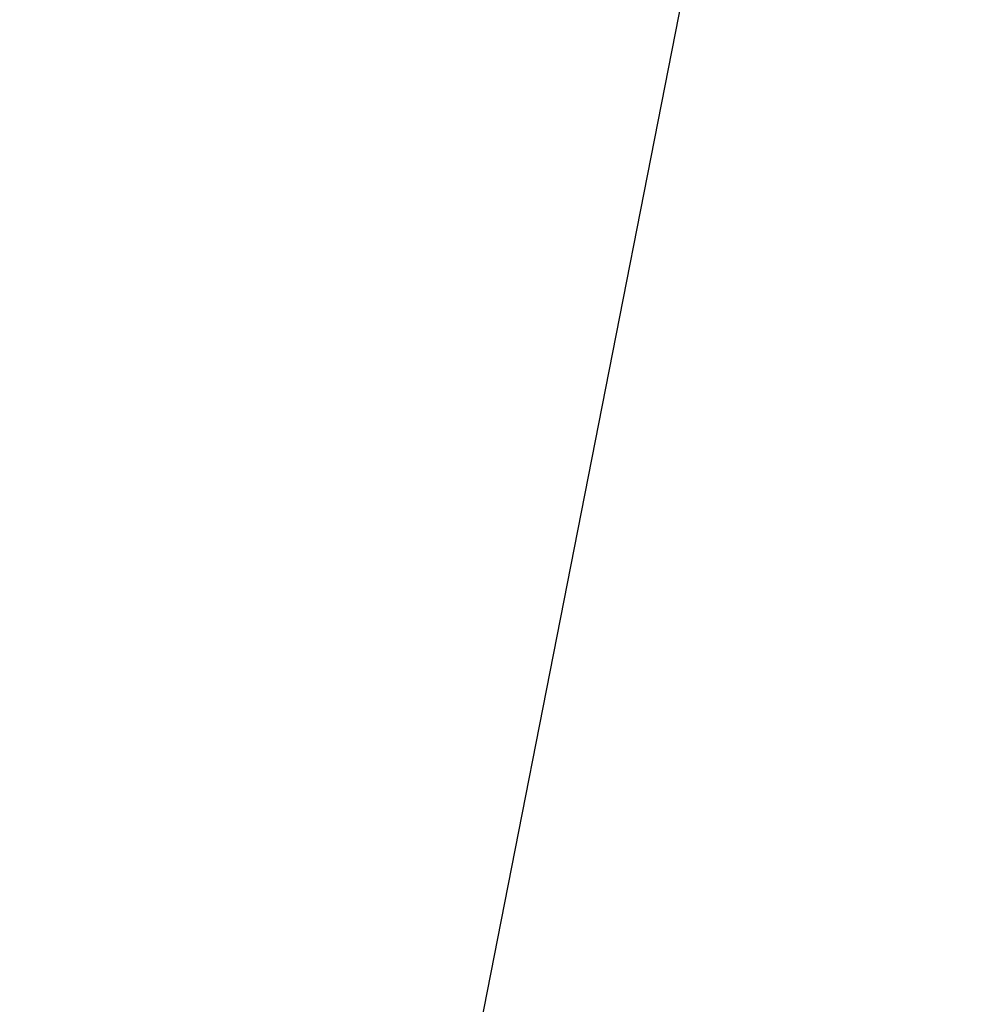
# Model space of a CAD drawing. Units: inches. Extents: x 3590 to 5167, y 65 to 1917.
# Tile 80 of 100: x 5050.6581 to 5051.162, y 1788.0928 to 1788.6144. Entities that reach past the tile are written whole.
import ezdxf

# ---------------------------------------------------------------- set-up
doc = ezdxf.new("R2010")
doc.units = ezdxf.units.IN
doc.layers.add('A-ANNO-DIMS', color=2, linetype='Continuous', lineweight=18)
doc.layers.add('L-PLNT', color=94, linetype='Continuous', lineweight=18)
doc.layers.add('DIENHOA', color=3, linetype='Continuous')
doc.styles.get("Standard").update_dxf_attribs({"font": 'arial.ttf'})
doc.dimstyles.new('ISO-25', dxfattribs={"dimtxt": 9, "dimasz": 2.5, "dimexe": 1.25, "dimexo": 0.625, "dimtad": 1, "dimdec": 1, "dimlunit": 3, "dimtxsty": 'Standard', "dimcen": 2.5, "dimadec": 0, "dimazin": 0, "dimtfac": 1, "dimtdec": 1, "dimtmove": 0, "dimatfit": 3, "dimfxl": 1, "dimarcsym": 0})

# ---------------------------------------------------------------- blocks, each defined once
blk = doc.blocks.new('Cay03_mb')
at = {"layer": 'DIENHOA'}
blk.add_line((9.944, 295.252), (25.486, 374.333), dxfattribs=at)
blk = doc.blocks.new('*D322')
at = {"layer": 'A-ANNO-DIMS', "color": 0, "lineweight": -2, "transparency": 16777216}
for p, q in [((5035.74373, 1766.18424), (5035.74373, 1761.19899)), ((5064.81203, 1766.18424), (5064.81203, 1761.19899)), ((5038.24373, 1762.44899), (5062.31203, 1762.44899)), ((5064.81203, 1762.44899), (5166.99109, 1762.44899))]:
    blk.add_line(p, q, dxfattribs=at)
at = {"layer": 'A-ANNO-DIMS', "color": 0, "transparency": 16777216}
for points in [[(5038.24373, 1762.86566), (5038.24373, 1762.03233), (5035.74373, 1762.44899)], [(5062.31203, 1762.86566), (5062.31203, 1762.03233), (5064.81203, 1762.44899)]]:
    blk.add_solid(points, dxfattribs=at)
at = {"layer": 'Defpoints', "color": 0, "transparency": 16777216}
for p in [(5035.74373, 1766.80924), (5064.81203, 1766.80924), (5064.81203, 1762.44899)]:
    blk.add_point(p, dxfattribs=at)
at = {"layer": 'A-ANNO-DIMS', "color": 0, "transparency": 16777216, "insert": (5117.15156, 1767.66915), "char_height": 9, "attachment_point": 5}
blk.add_mtext('PLANT 2\'-5" TYP.', dxfattribs=at)

msp = doc.modelspace()

# ---------------------------------------------------------------- block references
at = {"layer": 'L-PLNT', "xscale": 0.0245452446402784, "yscale": 0.0245452446402784, "zscale": 0.0245452446402784}
msp.add_blockref('Cay03_mb', (5050.43062, 1779.67584), dxfattribs=at)

# ---------------------------------------------------------------- dimensions: what is measured, and where the dimension line sits
at = {"layer": 'A-ANNO-DIMS'}
dim = msp.add_linear_dim(base=(5064.81203, 1762.44899), p1=(5035.74373, 1766.80924), p2=(5064.81203, 1766.80924), text='PLANT <> TYP.', dimstyle='ISO-25', override={"dimdec": 1, "dimlfac": 1, "dimrnd": 0, "dimzin": 1, "dimdsep": 46, "dimlunit": 4, "dimfrac": 2}, dxfattribs=at)
dim.commit()
dim.dimension.update_dxf_attribs({"geometry": '*D322', "text_midpoint": (5117.15156, 1767.66915)})

doc.saveas('drawing.dxf')
